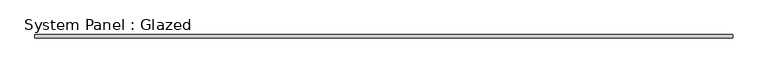
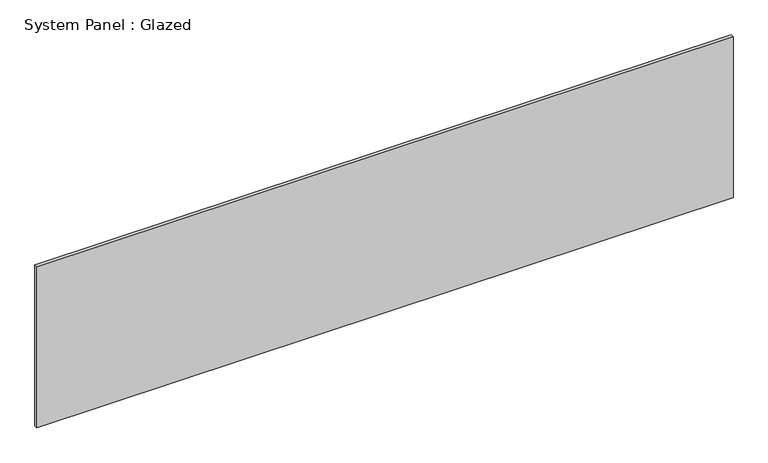
"""IFC4 building model written with IfcOpenShell, lengths in millimetres: plate geometry, System Panel : Glazed."""

from ifc_helpers import new_model, si_unit, origin, origin_with_axes, place, context, project, spatial, polyline, outline, extrude, source, transform, mapped, element, save


def system_panel_glazed_8bf14ce2(model_context):
    return source(origin(), model_context, "Body", "SweptSolid", [
        extrude(outline(polyline([(2495.55, 19.05), (-2495.55, 19.05), (-2495.55, 44.45), (2495.55, 44.45), (2495.55, 19.05)])), origin_with_axes(), (0.0, 0.0, 1.0), 1219.2),
    ])


if __name__ == "__main__":
    model = new_model("IFC4")
    model_context = context("Model", 3, world=origin())
    ifc_project = project(units=[si_unit("LENGTHUNIT", "METRE", prefix="MILLI")], contexts=[model_context])
    site = spatial("IfcSite", under=ifc_project)
    building = spatial("IfcBuilding", under=site)
    placement = place(None, origin())
    system_panel_glazed_shape = system_panel_glazed_8bf14ce2(model_context)
    element("IfcPlate", 1, ObjectType="System Panel : Glazed", at=placement, inside=building, context=model_context, shape_type="MappedRepresentation", body=[
        mapped(system_panel_glazed_shape, transform((0.0, 0.0, 0.0), x_axis=(1.0, 0.0, 0.0), y_axis=(0.0, 1.0, 0.0), z_axis=(0.0, 0.0, 1.0))),
    ])
    save(model, "model.ifc")

# Revit data of these elements
# Type "System Panel : Glazed"
#   Construction Type Id = "GSP4R"
#   Analytic Construction = "1/8 in Pilkington single glazing"
#   Visual Light Transmittance = 0.9
#   Solar Heat Gain Coefficient = 0.86
#   Heat Transfer Coefficient (U) = 1.18115 BTU/(h·ft²·°F)
# Element 1 (IfcPlate, "System Panel : Glazed")
#   Materials on its faces: "Glass"
# Materials
#   "Glass": class "Glass", colour RGB 0 128 192, transparency 0.75, Description = "Soda Lime Glass", Cost = 0
